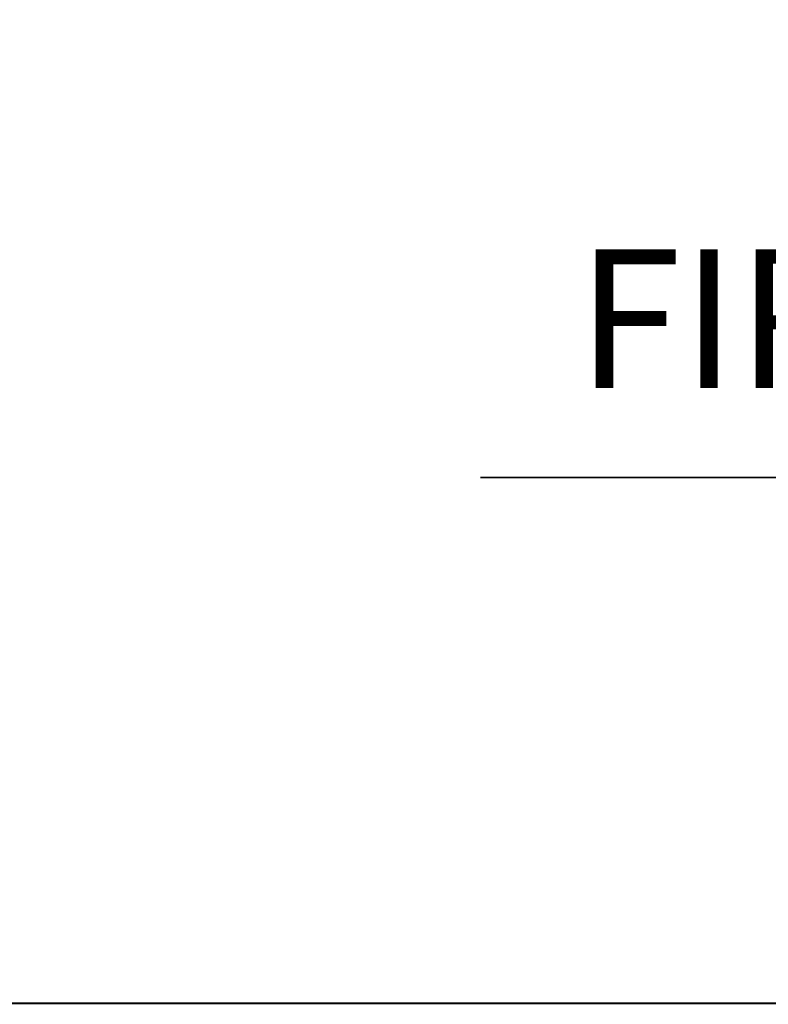
# Model space of a CAD drawing. Units: inches. Extents: x 1885 to 2748, y 783 to 2421.
# Tile 12 of 117: x 2065 to 2163, y 922 to 1050. Entities that reach past the tile are written whole.
import ezdxf

# ---------------------------------------------------------------- set-up
doc = ezdxf.new("R2010")
doc.units = ezdxf.units.IN
doc.layers.add('A-ANNO-DIMS', color=2, linetype='Continuous', lineweight=18)
doc.layers.add('A-ANNO-TTLB', color=7, linetype='Continuous', lineweight=35)
doc.styles.get("Standard").update_dxf_attribs({"font": 'arial.ttf'})
doc.dimstyles.get("Standard").update_dxf_attribs({"dimtxt": 0.18, "dimasz": 0.18, "dimexe": 0.18, "dimexo": 0.0625, "dimgap": 0.09, "dimtad": 0, "dimtih": 1, "dimtoh": 1, "dimdec": 4, "dimzin": 0, "dimdsep": 46, "dimtxsty": 'Standard', "dimcen": 0.09, "dimadec": 0, "dimazin": 0, "dimtfac": 1, "dimtdec": 4, "dimtofl": 0, "dimtmove": 0, "dimatfit": 3, "dimfxl": 1, "dimtolj": 1, "dimtzin": 0, "dimarcsym": 0})

# ---------------------------------------------------------------- blocks, each defined once
blk = doc.blocks.new('*D43')
at = {"layer": 'A-ANNO-DIMS', "color": 0, "lineweight": -2, "transparency": 16777216}
for p, q in [((1971.27, 1057.44), (1971.27, 922.48)), ((2618.27, 1057.44), (2618.27, 922.48)), ((1971.45, 922.66), (2294.48, 922.66)), ((2618.09, 922.66), (2295.06, 922.66))]:
    blk.add_line(p, q, dxfattribs=at)
at = {"layer": 'A-ANNO-DIMS', "color": 0, "transparency": 16777216}
for points in [[(1971.45, 922.69), (1971.45, 922.63), (1971.27, 922.66)], [(2618.09, 922.69), (2618.09, 922.63), (2618.27, 922.66)]]:
    blk.add_solid(points, dxfattribs=at)
at = {"layer": 'Defpoints', "color": 0, "transparency": 16777216}
for p in [(1971.27, 1057.51), (2618.27, 1057.51), (2618.27, 922.66)]:
    blk.add_point(p, dxfattribs=at)
at = {"layer": 'A-ANNO-DIMS', "color": 0, "transparency": 16777216, "insert": (2294.77, 922.66), "char_height": 0.18, "attachment_point": 5}
blk.add_mtext('\\A1;647', dxfattribs=at)

msp = doc.modelspace()

# ---------------------------------------------------------------- linework, layer by layer
at = {"layer": 'A-ANNO-TTLB'}
msp.add_line((2125.16, 990.91), (2382.12, 990.91), dxfattribs=at)
msp.add_lwpolyline([(1885.16, 2409.17), (2748.2, 2409.17), (2748.2, 922.58), (1885.16, 922.58)], close=True, dxfattribs=at)

# ---------------------------------------------------------------- texts
at = {"layer": 'A-ANNO-TTLB', "insert": (2137.65, 1020.52), "char_height": 18, "attachment_point": 1}
msp.add_mtext_dynamic_manual_height_columns('FIRST FLOOR PLAN', width=362.1951, gutter_width=12.5, heights=[0], dxfattribs=at)

# ---------------------------------------------------------------- dimensions: what is measured, and where the dimension line sits
at = {"layer": 'A-ANNO-DIMS'}
dim = msp.add_linear_dim(base=(2618.27, 922.66), p1=(1971.27, 1057.51), p2=(2618.27, 1057.51), dimstyle='Standard', override={"dimdec": 0, "dimlfac": 1, "dimrnd": 0, "dimzin": 0, "dimdsep": 46, "dimlunit": 2}, dxfattribs=at)
dim.commit()
dim.dimension.update_dxf_attribs({"geometry": '*D43', "text_midpoint": (2294.77, 922.66)})

doc.saveas('drawing.dxf')
